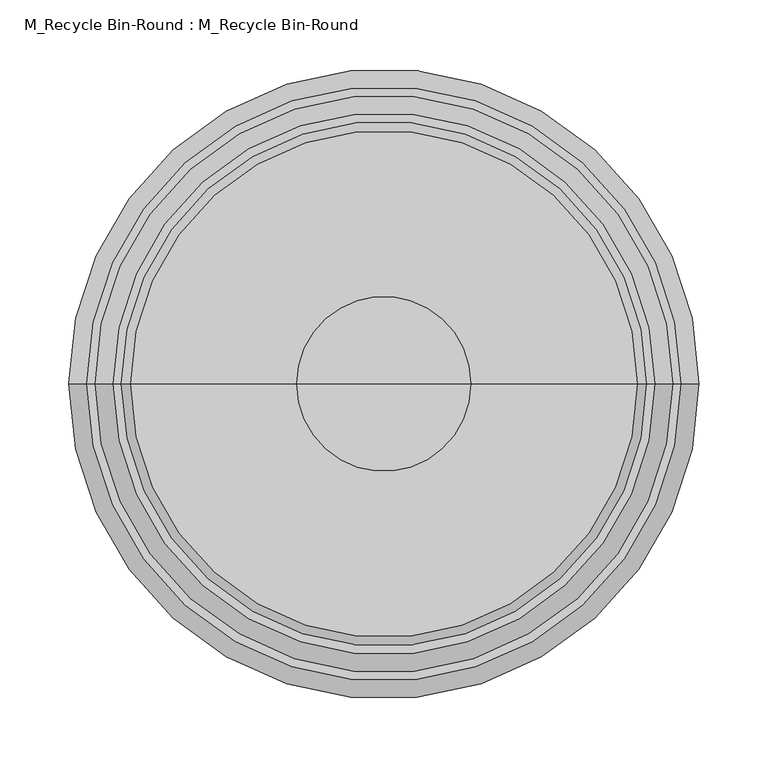
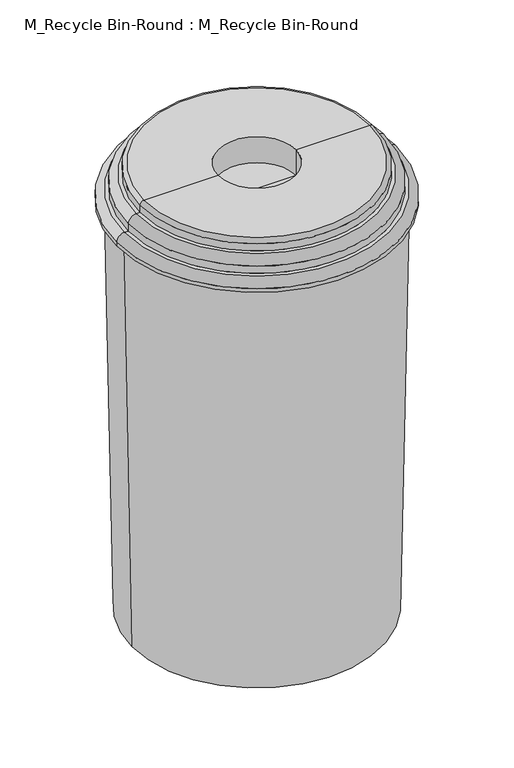
"""IFC4 building model written with IfcOpenShell, lengths in millimetres: proxy geometry, M_Recycle Bin-Round : M_Recycle Bin-Round."""

from ifc_helpers import new_model, si_unit, point, frame, origin, place, context, project, spatial, polyline, circle_curve, ellipse_curve, trimmed, source, transform, mapped, element, save
from ifc_brep_helpers import plane_surface, cylinder_surface, revolved_surface, advanced_brep


def m_recycle_bin_round_m_recycle_bin_round_6e7ed866(model_context):
    return source(origin(), model_context, "Body", "AdvancedBrep", [
        advanced_brep(
        [(-215.9, 0.0, 698.5), (215.9, 0.0, 698.5), (-203.2, 0.0, 0.0), (203.2, 0.0, 0.0)],
        [
            (0, 1, circle_curve(frame((0.0, 0.0, 698.5), z_axis=(0.0, 0.0, 1.0), x_axis=(-1.0, 0.0, 0.0)), 215.9)),
            (1, 0, circle_curve(frame((0.0, 0.0, 698.5), z_axis=(0.0, 0.0, 1.0), x_axis=(1.0, 0.0, 0.0)), 215.9)),
            (2, 3, circle_curve(frame((0.0, 0.0, 0.0), z_axis=(0.0, 0.0, -1.0), x_axis=(1.0, 0.0, 0.0)), 203.2)),
            (3, 2, circle_curve(frame((0.0, 0.0, 0.0), z_axis=(0.0, 0.0, -1.0), x_axis=(-1.0, 0.0, 0.0)), 203.2)),
            (3, 1),
            (0, 2),
        ],
        [
            plane_surface(frame((0.0, 0.0, 698.5), z_axis=(0.0, 0.0, 1.0), x_axis=(0.0, -1.0, 0.0))),
            plane_surface(frame((0.0, 0.0, 0.0), z_axis=(0.0, 0.0, -1.0), x_axis=(0.0, -1.0, 0.0))),
            revolved_surface(polyline([(203.2, 0.0, 0.0), (215.9, 0.0, 698.5)]), (0.0, 0.0, -11176.0), (0.0, 0.0, 1.0)),
            revolved_surface(polyline([(-203.2, 0.0, 0.0), (-215.9, 0.0, 698.5)]), (0.0, 0.0, -11176.0), (0.0, 0.0, 1.0)),
        ],
        [
            (0, [[1, 2]]),
            (1, [[3, 4]]),
            (2, [[-4, 5, -1, 6]]),
            (3, [[-3, -6, -2, -5]]),
        ],
    ),
        advanced_brep(
        [(-228.6, 0.0, 704.85), (228.6, 0.0, 704.85), (228.6, 0.0, 698.5), (-228.6, 0.0, 698.5), (-215.9, 0.0, 717.55), (215.9, 0.0, 717.55), (-209.55, 0.0, 717.55), (209.55, 0.0, 717.55), (-209.55, 0.0, 730.25), (209.55, 0.0, 730.25), (-196.85, 0.0, 742.95), (196.85, 0.0, 742.95), (-190.5, 0.0, 742.95), (190.5, 0.0, 742.95), (-190.5, 0.0, 755.65), (190.5, 0.0, 755.65), (-184.15, 0.0, 762.0), (184.15, 0.0, 762.0), (-63.5, 0.0, 762.0), (63.5, 0.0, 762.0), (-63.5, 0.0, 717.55), (63.5, 0.0, 717.55), (0.0, 0.0, 717.55), (0.0, 0.0, 698.5)],
        [
            (0, 1, circle_curve(frame((0.0, 0.0, 704.85), z_axis=(0.0, 0.0, -1.0), x_axis=(1.0, 0.0, 0.0)), 228.6)),
            (1, 2),
            (2, 3, circle_curve(frame((0.0, 0.0, 698.5), z_axis=(0.0, 0.0, 1.0), x_axis=(1.0, 0.0, 0.0)), 228.6)),
            (3, 0),
            (1, 0, circle_curve(frame((0.0, 0.0, 704.85), z_axis=(0.0, 0.0, -1.0), x_axis=(1.0, 0.0, 0.0)), 228.6)),
            (3, 2, circle_curve(frame((0.0, 0.0, 698.5), z_axis=(0.0, 0.0, 1.0), x_axis=(1.0, 0.0, 0.0)), 228.6)),
            (4, 5, circle_curve(frame((0.0, 0.0, 717.55), z_axis=(0.0, 0.0, -1.0), x_axis=(1.0, 0.0, 0.0)), 215.9)),
            (5, 1, circle_curve(frame((215.9, 0.0, 704.85), z_axis=(0.0, 1.0, 0.0), x_axis=(1.0, 0.0, 0.0)), 12.7)),
            (0, 4, circle_curve(frame((-215.9, 0.0, 704.85), z_axis=(0.0, 1.0, 0.0), x_axis=(-1.0, 0.0, 0.0)), 12.7)),
            (5, 4, circle_curve(frame((0.0, 0.0, 717.55), z_axis=(0.0, 0.0, -1.0), x_axis=(1.0, 0.0, 0.0)), 215.9)),
            (6, 7, circle_curve(frame((0.0, 0.0, 717.55), z_axis=(0.0, 0.0, -1.0), x_axis=(1.0, 0.0, 0.0)), 209.55)),
            (7, 5),
            (4, 6),
            (7, 6, circle_curve(frame((0.0, 0.0, 717.55), z_axis=(0.0, 0.0, -1.0), x_axis=(1.0, 0.0, 0.0)), 209.55)),
            (8, 9, circle_curve(frame((0.0, 0.0, 730.25), z_axis=(0.0, 0.0, -1.0), x_axis=(1.0, 0.0, 0.0)), 209.55)),
            (9, 7),
            (6, 8),
            (9, 8, circle_curve(frame((0.0, 0.0, 730.25), z_axis=(0.0, 0.0, -1.0), x_axis=(1.0, 0.0, 0.0)), 209.55)),
            (10, 11, circle_curve(frame((0.0, 0.0, 742.95), z_axis=(0.0, 0.0, -1.0), x_axis=(1.0, 0.0, 0.0)), 196.85)),
            (11, 9, circle_curve(frame((196.85, 0.0, 730.25), z_axis=(0.0, 1.0, 0.0), x_axis=(1.0, 0.0, 0.0)), 12.7)),
            (8, 10, circle_curve(frame((-196.85, 0.0, 730.25), z_axis=(0.0, 1.0, 0.0), x_axis=(-1.0, 0.0, 0.0)), 12.7)),
            (11, 10, circle_curve(frame((0.0, 0.0, 742.95), z_axis=(0.0, 0.0, -1.0), x_axis=(1.0, 0.0, 0.0)), 196.85)),
            (12, 13, circle_curve(frame((0.0, 0.0, 742.95), z_axis=(0.0, 0.0, -1.0), x_axis=(1.0, 0.0, 0.0)), 190.5)),
            (13, 11),
            (10, 12),
            (13, 12, circle_curve(frame((0.0, 0.0, 742.95), z_axis=(0.0, 0.0, -1.0), x_axis=(1.0, 0.0, 0.0)), 190.5)),
            (14, 15, circle_curve(frame((0.0, 0.0, 755.65), z_axis=(0.0, 0.0, -1.0), x_axis=(1.0, 0.0, 0.0)), 190.5)),
            (15, 13),
            (12, 14),
            (15, 14, circle_curve(frame((0.0, 0.0, 755.65), z_axis=(0.0, 0.0, -1.0), x_axis=(1.0, 0.0, 0.0)), 190.5)),
            (16, 17, circle_curve(frame((0.0, 0.0, 762.0), z_axis=(0.0, 0.0, -1.0), x_axis=(1.0, 0.0, 0.0)), 184.15)),
            (17, 15, circle_curve(frame((184.15, 0.0, 755.65), z_axis=(0.0, 1.0, 0.0), x_axis=(1.0, 0.0, 0.0)), 6.35)),
            (14, 16, circle_curve(frame((-184.15, 0.0, 755.65), z_axis=(0.0, 1.0, 0.0), x_axis=(-1.0, 0.0, 0.0)), 6.35)),
            (17, 16, circle_curve(frame((0.0, 0.0, 762.0), z_axis=(0.0, 0.0, -1.0), x_axis=(1.0, 0.0, 0.0)), 184.15)),
            (18, 19, circle_curve(frame((0.0, 0.0, 762.0), z_axis=(0.0, 0.0, -1.0), x_axis=(1.0, 0.0, 0.0)), 63.5)),
            (19, 17),
            (16, 18),
            (19, 18, circle_curve(frame((0.0, 0.0, 762.0), z_axis=(0.0, 0.0, -1.0), x_axis=(1.0, 0.0, 0.0)), 63.5)),
            (20, 21, circle_curve(frame((0.0, 0.0, 717.55), z_axis=(0.0, 0.0, -1.0), x_axis=(1.0, 0.0, 0.0)), 63.5)),
            (21, 19),
            (18, 20),
            (21, 20, circle_curve(frame((0.0, 0.0, 717.55), z_axis=(0.0, 0.0, -1.0), x_axis=(1.0, 0.0, 0.0)), 63.5)),
            (22, 21),
            (20, 22),
            (2, 23),
            (23, 3),
        ],
        [
            cylinder_surface(frame((0.0, 0.0, 698.5), z_axis=(0.0, 0.0, 1.0), x_axis=(1.0, 0.0, 0.0)), 228.6),
            revolved_surface(trimmed(ellipse_curve(frame((215.9, 0.0, 704.85), z_axis=(0.0, -1.0, 0.0), x_axis=(1.0, 0.0, 0.0)), 12.7, 12.7), [point((228.6, 0.0, 704.85))], [point((215.9, 0.0, 717.55))], True, "CARTESIAN"), (0.0, 0.0, 698.5), (0.0, 0.0, 1.0)),
            plane_surface(frame((0.0, 0.0, 717.55), z_axis=(0.0, 0.0, 1.0), x_axis=(1.0, 0.0, 0.0))),
            cylinder_surface(frame((0.0, 0.0, 698.5), z_axis=(0.0, 0.0, 1.0), x_axis=(1.0, 0.0, 0.0)), 209.55),
            revolved_surface(trimmed(ellipse_curve(frame((196.85, 0.0, 730.25), z_axis=(0.0, -1.0, 0.0), x_axis=(1.0, 0.0, 0.0)), 12.7, 12.7), [point((209.55, 0.0, 730.25))], [point((196.85, 0.0, 742.95))], True, "CARTESIAN"), (0.0, 0.0, 698.5), (0.0, 0.0, 1.0)),
            plane_surface(frame((0.0, 0.0, 742.95), z_axis=(0.0, 0.0, 1.0), x_axis=(1.0, 0.0, 0.0))),
            cylinder_surface(frame((0.0, 0.0, 698.5), z_axis=(0.0, 0.0, 1.0), x_axis=(1.0, 0.0, 0.0)), 190.5),
            revolved_surface(trimmed(ellipse_curve(frame((184.15, 0.0, 755.65), z_axis=(0.0, -1.0, 0.0), x_axis=(1.0, 0.0, 0.0)), 6.35, 6.35), [point((190.5, 0.0, 755.65))], [point((184.15, 0.0, 762.0))], True, "CARTESIAN"), (0.0, 0.0, 698.5), (0.0, 0.0, 1.0)),
            plane_surface(frame((0.0, 0.0, 762.0), z_axis=(0.0, 0.0, 1.0), x_axis=(1.0, 0.0, 0.0))),
            revolved_surface(polyline([(63.5, 0.0, 762.0), (63.5, 0.0, 717.55)]), (0.0, 0.0, 698.5), (0.0, 0.0, 1.0)),
            plane_surface(frame((0.0, 0.0, 698.5), z_axis=(0.0, 0.0, -1.0), x_axis=(1.0, 0.0, 0.0))),
        ],
        [
            (0, [[1, 2, 3, 4]]),
            (0, [[5, -4, 6, -2]]),
            (1, [[7, 8, -1, 9]]),
            (1, [[10, -9, -5, -8]]),
            (2, [[11, 12, -7, 13]]),
            (2, [[14, -13, -10, -12]]),
            (3, [[15, 16, -11, 17]]),
            (3, [[18, -17, -14, -16]]),
            (4, [[19, 20, -15, 21]]),
            (4, [[22, -21, -18, -20]]),
            (5, [[23, 24, -19, 25]]),
            (5, [[26, -25, -22, -24]]),
            (6, [[27, 28, -23, 29]]),
            (6, [[30, -29, -26, -28]]),
            (7, [[31, 32, -27, 33]]),
            (7, [[34, -33, -30, -32]]),
            (8, [[35, 36, -31, 37]]),
            (8, [[38, -37, -34, -36]]),
            (9, [[39, 40, -35, 41]]),
            (9, [[42, -41, -38, -40]]),
            (2, [[43, -39, 44]]),
            (2, [[-44, -42, -43]]),
            (10, [[-3, 45, 46]]),
            (10, [[-6, -46, -45]]),
        ],
    ),
    ])


if __name__ == "__main__":
    model = new_model("IFC4")
    model_context = context("Model", 3, world=origin())
    ifc_project = project(units=[si_unit("LENGTHUNIT", "METRE", prefix="MILLI")], contexts=[model_context])
    site = spatial("IfcSite", under=ifc_project)
    building = spatial("IfcBuilding", under=site)
    placement = place(None, origin())
    m_recycle_bin_round_m_recycle_bin_round_shape = m_recycle_bin_round_m_recycle_bin_round_6e7ed866(model_context)
    element("IfcBuildingElementProxy", 1, Name="M_Recycle Bin-Round : M_Recycle Bin-Round", ObjectType="M_Recycle Bin-Round : M_Recycle Bin-Round", at=placement, inside=building, context=model_context, shape_type="MappedRepresentation", body=[
        mapped(m_recycle_bin_round_m_recycle_bin_round_shape, transform((0.0, 0.0, 0.0), x_axis=(1.0, 0.0, 0.0), y_axis=(0.0, 1.0, 0.0), z_axis=(0.0, 0.0, 1.0))),
    ])
    save(model, "model.ifc")

# Revit data of these elements
# Type "M_Recycle Bin-Round : M_Recycle Bin-Round"
#   Default Elevation = 0
# Element 1 (IfcBuildingElementProxy, "M_Recycle Bin-Round : M_Recycle Bin-Round")
#   Materials on its faces: "Plastic - Blue", "Default - Black"
# Materials
#   "Plastic - Blue": class "Plastic", colour RGB 0 0 212, transparency 0
#   "Default - Black": colour RGB 0 0 0, transparency 0
